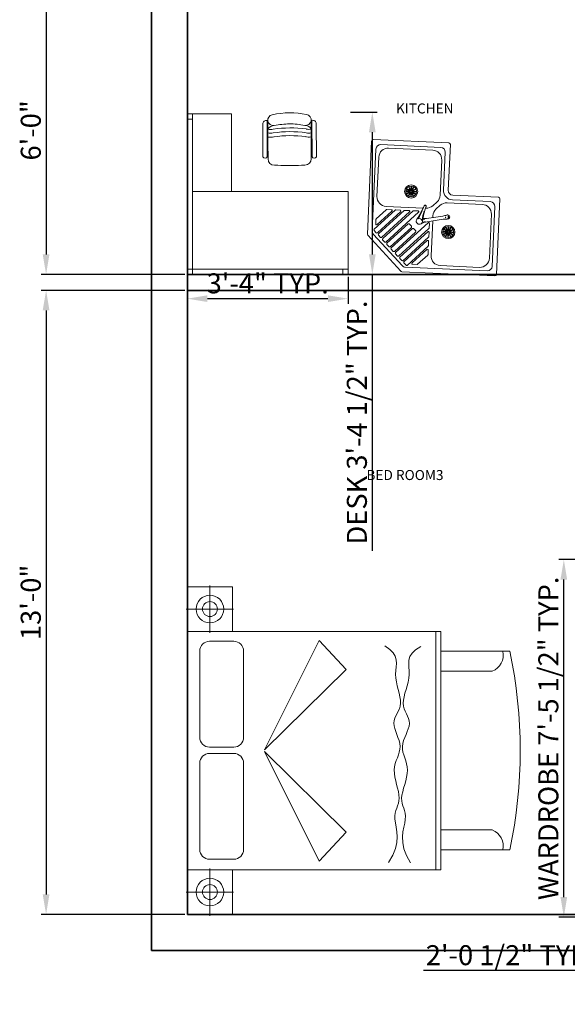
# Model space of a CAD drawing. Units: inches. Extents: x -24887 to 3061, y 1794 to 4919553.
# Tile 8 of 14: x 2721 to 2858, y 1943 to 2190. Entities that reach past the tile are written whole.
import ezdxf

# ---------------------------------------------------------------- set-up
doc = ezdxf.new("R2010")
doc.units = ezdxf.units.IN
for name, color, linetype, lineweight in [('A-ANNO-DIMS', 2, 'Continuous', 18), ('A-AREA-IDEN', 7, 'Continuous', 18), ('A-FLOR-FIXT', 9, 'Continuous', 18), ('A-FURN', 8, 'Continuous', 18), ('wall', 7, 'Continuous', 35)]:
    doc.layers.add(name, color=color, linetype=linetype, lineweight=lineweight)
doc.styles.get("Standard").update_dxf_attribs({"font": 'arial.ttf'})
doc.dimstyles.new('ISO-25', dxfattribs={"dimtxt": 5, "dimasz": 5, "dimexe": 1.25, "dimexo": 0.625, "dimtad": 1, "dimdec": 1, "dimlunit": 3, "dimtxsty": 'Standard', "dimcen": 2.5, "dimadec": 0, "dimazin": 0, "dimtfac": 1, "dimtdec": 1, "dimtmove": 0, "dimatfit": 3, "dimfxl": 1, "dimarcsym": 0})

# ---------------------------------------------------------------- blocks, each defined once
blk = doc.blocks.new('A$C4F543DC7')
for p, q in [((0.0134, 3.35, -0.1688), (3.3134, 3.35, -0.1688)), ((0.4634, 3.35, -0.1688), (0.0134, 3.35, -0.1688)), ((0.0134, 2.896, -0.1688), (0.0134, 3.35, -0.1688)), ((0.0134, 3.35, -0.1688), (0.0134, 2.896, -0.1688)), ((0.2381, 3.1233, -0.4388), (0.2381, 3.3614, -0.4388)), ((0.4634, 3.35, -0.1688), (0.4634, 0.8, -0.1688)), ((2.8634, 3.35, -0.1688), (0.4634, 3.35, -0.1688)), ((0.4634, 2.896, -0.1688), (0.4634, 3.35, -0.1688)), ((2.8634, 0.8, -0.1688), (2.8634, 3.35, -0.1688)), ((2.8634, 3.35, -0.1688), (3.3134, 3.35, -0.1688)), ((2.8634, 2.896, -0.1688), (2.8634, 3.35, -0.1688)), ((3.0888, 3.1233, -0.4388), (3.0888, 3.3614, -0.4388)), ((3.3134, 3.35, -0.1688), (3.3134, 2.896, -0.1688)), ((3.3134, 3.35, -0.1688), (3.3134, 2.896, -0.1688)), ((1.5354, 3.226, -0.1688), (0.6684, 3.226, -0.1688)), ((2.6644, 3.226, -0.1688), (1.7974, 3.226, -0.1688)), ((0.2381, 3.1233, -0.4388), (0, 3.1233, -0.4388)), ((0.2381, 3.1233, -0.4388), (0.4762, 3.1233, -0.4388)), ((0.2381, 3.1233, -0.4388), (0.2381, 2.8852, -0.4388)), ((0.5684, 3.126, -0.1688), (0.5684, 2.884, -0.1688)), ((1.6354, 2.884, -0.1688), (1.6354, 3.126, -0.1688)), ((1.6974, 3.126, -0.1688), (1.6974, 2.884, -0.1688)), ((2.7644, 2.884, -0.1688), (2.7644, 3.126, -0.1688)), ((3.0888, 3.1233, -0.4388), (2.8507, 3.1233, -0.4388)), ((3.0888, 3.1233, -0.4388), (3.0888, 2.8852, -0.4388)), ((3.0888, 3.1233, -0.4388), (3.3269, 3.1233, -0.4388)), ((0.4634, 2.896, -0.1688), (0.0134, 2.896, -0.1688)), ((0.0134, 2.896, -0.1688), (0.4634, 2.896, -0.1688)), ((0.4634, 0.8, -0.1688), (0.4634, 2.896, -0.1688)), ((2.8634, 2.896, -0.1688), (2.8634, 0.8, -0.1688)), ((3.3134, 2.896, -0.1688), (2.8634, 2.896, -0.1688)), ((3.3134, 2.896, -0.1688), (2.8634, 2.896, -0.1688)), ((0.6684, 2.784, -0.1688), (1.5354, 2.784, -0.1688)), ((1.7974, 2.784, -0.1688), (2.6644, 2.784, -0.1688)), ((1.6534, 2.573, -0.1688), (0.5504, 2.025, -0.1688)), ((0.8414, 1.752, -0.1688), (1.6534, 2.573, -0.1688)), ((2.4814, 1.752, -0.1688), (1.6694, 2.573, -0.1688)), ((1.6694, 2.573, -0.1688), (2.7724, 2.025, -0.1688)), ((0.5504, 2.025, -0.1688), (0.8414, 1.752, -0.1688)), ((2.7724, 2.025, -0.1688), (2.4814, 1.752, -0.1688)), ((0.5369, 1.3267, -0.1688), (0.6088, 1.2835, -0.1688)), ((2.6479, 1.2774, -0.1688), (2.683, 1.312, -0.1688)), ((2.683, 1.312, -0.1688), (2.7182, 1.3641, -0.1688)), ((0.6088, 1.2835, -0.1688), (0.6756, 1.2566, -0.1688)), ((0.6756, 1.2566, -0.1688), (0.7373, 1.2428, -0.1688)), ((0.7373, 1.2428, -0.1688), (0.794, 1.239, -0.1688)), ((0.794, 1.239, -0.1688), (0.8457, 1.242, -0.1688)), ((0.8457, 1.242, -0.1688), (0.8925, 1.2489, -0.1688)), ((0.8925, 1.2489, -0.1688), (0.9345, 1.2564, -0.1688)), ((0.9345, 1.2564, -0.1688), (0.9718, 1.2615, -0.1688)), ((0.9718, 1.2615, -0.1688), (1.0044, 1.2617, -0.1688)), ((1.0044, 1.2617, -0.1688), (1.0334, 1.2578, -0.1688)), ((1.0334, 1.2578, -0.1688), (1.0597, 1.2509, -0.1688)), ((1.0597, 1.2509, -0.1688), (1.0842, 1.2424, -0.1688)), ((1.0842, 1.2424, -0.1688), (1.1081, 1.2336, -0.1688)), ((1.1081, 1.2336, -0.1688), (1.1322, 1.2257, -0.1688)), ((1.1316, 1.1872, -0.1688), (1.1573, 1.192, -0.1688)), ((1.1322, 1.2257, -0.1688), (1.1577, 1.2201, -0.1688)), ((1.1573, 1.192, -0.1688), (1.1851, 1.1932, -0.1688)), ((1.1577, 1.2201, -0.1688), (1.1855, 1.218, -0.1688)), ((1.1851, 1.1932, -0.1688), (1.2158, 1.1898, -0.1688)), ((1.1855, 1.218, -0.1688), (1.2163, 1.2204, -0.1688)), ((1.2163, 1.2204, -0.1688), (1.2498, 1.2264, -0.1688)), ((1.2498, 1.2264, -0.1688), (1.2852, 1.2347, -0.1688)), ((1.2852, 1.2347, -0.1688), (1.3218, 1.2441, -0.1688)), ((1.3218, 1.2441, -0.1688), (1.3591, 1.2533, -0.1688)), ((1.3591, 1.2533, -0.1688), (1.3963, 1.2612, -0.1688)), ((1.3963, 1.2612, -0.1688), (1.4328, 1.2664, -0.1688)), ((1.4328, 1.2664, -0.1688), (1.4679, 1.2677, -0.1688)), ((1.4679, 1.2677, -0.1688), (1.501, 1.2643, -0.1688)), ((1.501, 1.2643, -0.1688), (1.5324, 1.257, -0.1688)), ((1.5324, 1.257, -0.1688), (1.5624, 1.2473, -0.1688)), ((1.5624, 1.2473, -0.1688), (1.5915, 1.2365, -0.1688)), ((1.5915, 1.2365, -0.1688), (1.6199, 1.2259, -0.1688)), ((1.6199, 1.2259, -0.1688), (1.6481, 1.2169, -0.1688)), ((1.6481, 1.2169, -0.1688), (1.6765, 1.2108, -0.1688)), ((1.6765, 1.2108, -0.1688), (1.7053, 1.209, -0.1688)), ((1.7053, 1.209, -0.1688), (1.7349, 1.2124, -0.1688)), ((1.7349, 1.2124, -0.1688), (1.7651, 1.2199, -0.1688)), ((1.7651, 1.2199, -0.1688), (1.7955, 1.2301, -0.1688)), ((1.7955, 1.2301, -0.1688), (1.8258, 1.2417, -0.1688)), ((1.8258, 1.2417, -0.1688), (1.8557, 1.2531, -0.1688)), ((1.8557, 1.2531, -0.1688), (1.8849, 1.263, -0.1688)), ((1.8849, 1.263, -0.1688), (1.913, 1.2698, -0.1688)), ((1.913, 1.2698, -0.1688), (1.9397, 1.2722, -0.1688)), ((1.9397, 1.2722, -0.1688), (1.9649, 1.2692, -0.1688)), ((1.9649, 1.2692, -0.1688), (1.989, 1.2617, -0.1688)), ((1.989, 1.2617, -0.1688), (2.0124, 1.2512, -0.1688)), ((2.0124, 1.2512, -0.1688), (2.0359, 1.2391, -0.1688)), ((2.0359, 1.2391, -0.1688), (2.0599, 1.2269, -0.1688)), ((2.0599, 1.2269, -0.1688), (2.0849, 1.216, -0.1688)), ((2.0849, 1.216, -0.1688), (2.1117, 1.2077, -0.1688)), ((2.1117, 1.2077, -0.1688), (2.1407, 1.2037, -0.1688)), ((2.1407, 1.2037, -0.1688), (2.1723, 1.2047, -0.1688)), ((2.1723, 1.2047, -0.1688), (2.2062, 1.21, -0.1688)), ((2.2062, 1.21, -0.1688), (2.242, 1.2182, -0.1688)), ((2.242, 1.2182, -0.1688), (2.2791, 1.2279, -0.1688)), ((2.2791, 1.2279, -0.1688), (2.3173, 1.2378, -0.1688)), ((2.3173, 1.2378, -0.1688), (2.3558, 1.2465, -0.1688)), ((2.3558, 1.2465, -0.1688), (2.3944, 1.2527, -0.1688)), ((2.3944, 1.2527, -0.1688), (2.4325, 1.255, -0.1688)), ((2.4325, 1.255, -0.1688), (2.4698, 1.2529, -0.1688)), ((2.4698, 1.2529, -0.1688), (2.5064, 1.2488, -0.1688)), ((2.5064, 1.2488, -0.1688), (2.5423, 1.2459, -0.1688)), ((2.5423, 1.2459, -0.1688), (2.5777, 1.2476, -0.1688)), ((2.5777, 1.2476, -0.1688), (2.6129, 1.257, -0.1688)), ((2.6129, 1.257, -0.1688), (2.6479, 1.2774, -0.1688)), ((0.5334, 1.105, -0.1688), (0.6067, 1.1458, -0.1688)), ((0.6067, 1.1458, -0.1688), (0.6743, 1.1706, -0.1688)), ((0.6743, 1.1706, -0.1688), (0.7364, 1.1825, -0.1688)), ((0.7364, 1.1825, -0.1688), (0.7931, 1.1846, -0.1688)), ((0.7931, 1.1846, -0.1688), (0.8447, 1.1799, -0.1688)), ((0.8447, 1.1799, -0.1688), (0.8913, 1.1716, -0.1688)), ((0.8913, 1.1716, -0.1688), (0.9331, 1.1628, -0.1688)), ((0.9331, 1.1628, -0.1688), (0.9701, 1.1565, -0.1688)), ((0.9701, 1.1565, -0.1688), (1.0027, 1.1552, -0.1688)), ((1.0027, 1.1552, -0.1688), (1.0318, 1.1582, -0.1688)), ((1.0318, 1.1582, -0.1688), (1.0583, 1.1642, -0.1688)), ((1.0583, 1.1642, -0.1688), (1.0831, 1.172, -0.1688)), ((1.0831, 1.172, -0.1688), (1.1072, 1.18, -0.1688)), ((1.1072, 1.18, -0.1688), (1.1316, 1.1872, -0.1688)), ((1.2158, 1.1898, -0.1688), (1.2491, 1.1828, -0.1688)), ((1.2491, 1.1828, -0.1688), (1.2842, 1.1734, -0.1688)), ((1.2842, 1.1734, -0.1688), (1.3206, 1.1629, -0.1688)), ((1.3206, 1.1629, -0.1688), (1.3575, 1.1524, -0.1688)), ((1.3575, 1.1524, -0.1688), (1.3945, 1.1434, -0.1688)), ((1.3945, 1.1434, -0.1688), (1.4308, 1.1371, -0.1688)), ((1.4308, 1.1371, -0.1688), (1.4658, 1.1347, -0.1688)), ((1.4658, 1.1347, -0.1688), (1.499, 1.137, -0.1688)), ((1.499, 1.137, -0.1688), (1.5306, 1.1433, -0.1688)), ((1.5306, 1.1433, -0.1688), (1.5609, 1.152, -0.1688)), ((1.5609, 1.152, -0.1688), (1.5903, 1.1619, -0.1688)), ((1.5903, 1.1619, -0.1688), (1.6191, 1.1716, -0.1688)), ((1.6191, 1.1716, -0.1688), (1.6475, 1.1797, -0.1688)), ((1.6475, 1.1797, -0.1688), (1.676, 1.1849, -0.1688)), ((1.676, 1.1849, -0.1688), (1.7049, 1.1858, -0.1688)), ((1.7049, 1.1858, -0.1688), (1.7344, 1.1816, -0.1688)), ((1.7344, 1.1816, -0.1688), (1.7643, 1.1731, -0.1688)), ((1.7643, 1.1731, -0.1688), (1.7944, 1.1619, -0.1688)), ((1.7944, 1.1619, -0.1688), (1.8244, 1.1494, -0.1688)), ((1.8244, 1.1494, -0.1688), (1.8539, 1.137, -0.1688)), ((1.8539, 1.137, -0.1688), (1.8827, 1.1263, -0.1688)), ((1.8827, 1.1263, -0.1688), (1.9106, 1.1186, -0.1688)), ((1.9106, 1.1186, -0.1688), (1.9373, 1.1153, -0.1688)), ((1.9373, 1.1153, -0.1688), (1.9625, 1.1176, -0.1688)), ((1.9625, 1.1176, -0.1688), (1.9868, 1.1243, -0.1688)), ((1.9868, 1.1243, -0.1688), (2.0106, 1.134, -0.1688)), ((2.0106, 1.134, -0.1688), (2.0344, 1.1454, -0.1688)), ((2.0344, 1.1454, -0.1688), (2.0588, 1.1568, -0.1688)), ((2.0588, 1.1568, -0.1688), (2.0842, 1.167, -0.1688)), ((2.0842, 1.167, -0.1688), (2.1112, 1.1743, -0.1688)), ((2.1112, 1.1743, -0.1688), (2.1403, 1.1775, -0.1688)), ((2.1403, 1.1775, -0.1688), (2.1718, 1.1755, -0.1688)), ((2.1718, 1.1755, -0.1688), (2.2056, 1.1691, -0.1688)), ((2.2056, 1.1691, -0.1688), (2.2411, 1.1598, -0.1688)), ((2.2411, 1.1598, -0.1688), (2.2779, 1.1489, -0.1688)), ((2.2779, 1.1489, -0.1688), (2.3157, 1.1379, -0.1688)), ((2.3157, 1.1379, -0.1688), (2.354, 1.1279, -0.1688)), ((2.354, 1.1279, -0.1688), (2.3923, 1.1205, -0.1688)), ((2.3923, 1.1205, -0.1688), (2.4304, 1.117, -0.1688)), ((2.4304, 1.117, -0.1688), (2.4677, 1.118, -0.1688)), ((2.4677, 1.118, -0.1688), (2.5043, 1.1209, -0.1688)), ((2.5043, 1.1209, -0.1688), (2.5403, 1.1226, -0.1688)), ((2.5403, 1.1226, -0.1688), (2.5757, 1.1199, -0.1688)), ((2.5757, 1.1199, -0.1688), (2.6106, 1.1094, -0.1688)), ((2.6106, 1.1094, -0.1688), (2.645, 1.0879, -0.1688)), ((2.645, 1.0879, -0.1688), (2.6789, 1.0522, -0.1688)), ((2.6789, 1.0522, -0.1688), (2.7124, 0.999, -0.1688)), ((0.4634, 0.85, -0.1688), (2.8634, 0.85, -0.1688)), ((0.4634, 0.8, -0.1688), (2.8634, 0.8, -0.1688)), ((0.6634, 0.8, -0.1688), (0.4634, 0.8, -0.1688)), ((0.6634, 0.8, -0.1688), (2.6634, 0.8, -0.1688)), ((0.6634, 0.104, -0.1688), (0.6634, 0.8, -0.1688)), ((0.6634, 0.104, -0.1688), (0.6634, 0.8, -0.1688)), ((0.8634, 0.281, -0.1688), (0.8634, 0.8, -0.1688)), ((2.4634, 0.8, -0.1688), (2.4634, 0.281, -0.1688)), ((2.8634, 0.8, -0.1688), (2.6634, 0.8, -0.1688)), ((2.6634, 0.8, -0.1688), (2.6634, 0.104, -0.1688)), ((2.6634, 0.8, -0.1688), (2.6634, 0.104, -0.1688))]:
    blk.add_line(p, q)
for centre, radius in [((0.2381, 3.1233, -0.4388), 0.139), ((0.2381, 3.1233, -0.4388), 0.075), ((3.0888, 3.1233, -0.4388), 0.139), ((3.0888, 3.1233, -0.4388), 0.075)]:
    blk.add_circle(centre, radius)
for centre, radius, start, end in [((0.6684, 3.126, -0.1688), 0.1, 90, 180), ((1.5354, 3.126, -0.1688), 0.1, 0, 90), ((1.7974, 3.126, -0.1688), 0.1, 90, 180), ((2.6644, 3.126, -0.1688), 0.1, 0, 90), ((0.6684, 2.884, -0.1688), 0.1, 180, 270), ((1.5354, 2.884, -0.1688), 0.1, 270, 0), ((1.7974, 2.884, -0.1688), 0.1, 180, 270), ((2.6644, 2.884, -0.1688), 0.1, 270, 0), ((0.6994, 0.3472, -0.1688), 0.1769, 258.2616, 338.03196), ((2.6275, 0.3472, -0.1688), 0.1769, 201.96804, 281.7384), ((1.6634, 4.8597, -0.1688), 4.8597, 258.12517, 281.87483), ((1.6634, 4.8597, -0.1688), 4.8597, 258.12517, 281.87483)]:
    blk.add_arc(centre, radius, start, end)
blk = doc.blocks.new('A$C4E531579')
for p, q in [((222.1, 827.1), (2.9, 607.9)), ((229.1, 830), (820, 830)), ((830, 820), (830, 340)), ((228.6, 791.2), (38.8, 601.4)), ((225.6, 759.9), (211.5, 745.8)), ((388.5, 604.1), (232.7, 759.9)), ((253.9, 788.2), (239.8, 774.1)), ((381.5, 625.3), (239.8, 767)), ((249.9, 800), (770, 800)), ((388.5, 660.7), (261, 788.2)), ((381.5, 681.9), (291.9, 771.5)), ((295.4, 780), (323.7, 780)), ((388.5, 717.2), (327.2, 778.5)), ((720, 780), (470, 780)), ((800, 770), (800, 390)), ((169.1, 703.4), (154.9, 689.2)), ((305.1, 574.4), (176.1, 703.4)), ((197.4, 731.6), (183.2, 717.5)), ((381.5, 512.2), (183.2, 710.4)), ((388.5, 547.5), (204.4, 731.6)), ((381.5, 568.7), (211.5, 738.7)), ((390, 713.7), (390, 685.4)), ((410, 720), (410, 483.9)), ((780, 440), (780, 720)), ((98.4, 632.6), (112.5, 646.8)), ((282.5, 441.5), (98.4, 625.6)), ((317.8, 448.5), (119.6, 646.8)), ((126.6, 660.9), (140.8, 675.1)), ((255.6, 524.9), (126.6, 653.9)), ((276.8, 546.1), (147.9, 675.1)), ((283.9, 553.2), (154.9, 682.1)), ((390, 657.1), (390, 628.8)), ((0, 10), (0, 600.9)), ((30, 60), (30, 580.1)), ((41.8, 576.1), (55.9, 590.2)), ((169.3, 441.5), (41.8, 569)), ((204.7, 448.5), (63, 590.2)), ((70.1, 604.4), (84.2, 618.5)), ((225.9, 441.5), (70.1, 597.3)), ((261.3, 448.5), (91.3, 618.5)), ((305.1, 567.3), (291, 553.2)), ((390, 600.6), (390, 572.3)), ((50, 534.6), (50, 506.3)), ((112.8, 441.5), (51.5, 502.8)), ((148.1, 448.5), (58.5, 538.1)), ((262.7, 524.9), (276.8, 539)), ((390, 544), (390, 515.7)), ((116.3, 440), (144.6, 440)), ((172.9, 440), (201.2, 440)), ((229.4, 440), (257.7, 440)), ((286, 440), (314.3, 440)), ((344.7, 353.4), (324.5, 455.5)), ((344.5, 460.1), (364.9, 357.1)), ((410, 468.8), (410, 466.1)), ((110, 420), (331.5, 420)), ((352.4, 420), (363.9, 420)), ((406.4, 402.4), (432.4, 376.4)), ((427.6, 423.6), (453.6, 397.6)), ((496.1, 380), (720, 380)), ((50, 110), (50, 360)), ((450, 333.9), (450, 110)), ((530, 360), (770, 360)), ((530, 330), (820, 330)), ((470, 300), (470, 60)), ((500, 300), (500, 10)), ((440, 30), (60, 30)), ((390, 50), (110, 50)), ((490, 0), (10, 0))]:
    blk.add_line(p, q)
for centre, radius in [((511.9, 565), 41.9), ((511.9, 565), 34.4), ((511.9, 565), 5.37), ((265, 318.1), 41.9), ((265, 318.1), 34.4), ((265, 318.1), 5.37)]:
    blk.add_circle(centre, radius)
for centre, radius, start, end in [((229.1, 820), 10, 90, 135), ((820, 820), 10, 0, 90), ((229.2, 756.4), 5, 45, 135), ((249.9, 770), 30, 90, 135), ((243.3, 770.5), 5, 135, 225), ((257.5, 784.7), 5, 45, 135), ((295.4, 775), 5, 90, 225), ((323.7, 775), 5, 45, 90), ((470, 720), 60, 90, 180), ((720, 720), 60, 0, 90), ((770, 770), 30, 0, 90), ((158.5, 685.7), 5, 135, 225), ((172.6, 699.8), 5, 45, 135), ((186.7, 714), 5, 135, 225), ((200.9, 728.1), 5, 45, 135), ((215, 742.2), 5, 135, 225), ((385, 713.7), 5, 0, 45), ((101.9, 629.1), 5, 135, 225), ((116, 643.3), 5, 45, 135), ((130.2, 657.4), 5, 135, 225), ((144.3, 671.5), 5, 45, 135), ((385, 685.4), 5, 225, 0), ((385, 628.8), 5, 225, 0), ((385, 657.1), 5, 0, 45), ((10, 600.9), 10, 135, 180), ((60, 580.1), 30, 135, 180), ((45.3, 572.5), 5, 135, 225), ((59.5, 586.7), 5, 45, 135), ((73.6, 600.8), 5, 135, 225), ((87.8, 615), 5, 45, 135), ((301.6, 570.8), 5, 315, 45), ((385, 572.3), 5, 225, 0), ((385, 600.6), 5, 0, 45), ((55, 534.6), 5, 45, 180), ((55, 506.3), 5, 180, 225), ((259.2, 528.4), 5, 225, 315), ((273.3, 542.6), 5, 315, 45), ((287.4, 556.7), 5, 225, 315), ((325.6, 504.4), 20, 52.72293, 268.78568), ((326.2, 504.9), 16.2, 278.92915, 32.15573), ((583, 916.9), 466.4, 238.27092, 250.20216), ((479.5, 750.1), 274.6, 239.9645, 252.02573), ((385, 515.7), 5, 225, 0), ((385, 544), 5, 0, 45), ((116.3, 445), 5, 225, 270), ((144.6, 445), 5, 270, 45), ((172.9, 445), 5, 225, 270), ((201.2, 445), 5, 270, 45), ((229.4, 445), 5, 225, 270), ((257.7, 445), 5, 270, 45), ((286, 445), 5, 225, 270), ((226.1, 437.3), 100, 10.4867, 33.97381), ((314.3, 445), 5, 270, 45), ((296.1, 462.7), 29.3, 9.84672, 38.35374), ((282.9, 16.5), 469.7, 72.94476, 84.83287), ((305.7, 211.8), 277.4, 72.23491, 84.23498), ((368.8, 476.8), 29.3, 168.25085, 191.99309), ((442.8, 478.3), 100, 177.65932, 190.48676), ((470, 466.1), 60, 180, 225), ((422.7, 471.9), 6.64, 252.6444, 68.86421), ((420.8, 471.6), 4.91, 314.25167, 37.23492), ((720, 440), 60, 270, 0), ((110, 360), 60, 90, 180), ((363.9, 360), 60, 45, 90), ((390, 333.9), 60, 0, 45), ((496.1, 440), 60, 225, 270), ((770, 390), 30, 270, 0), ((246.4, 335.2), 100, 355.98426, 10.4867), ((360, 327.2), 13.9, 175.98426, 24.98921), ((359.8, 327.5), 8.12, 180.36355, 342.44433), ((359, 332), 7.59, 72.42297, 131.67578), ((463.2, 375.3), 100, 190.48676, 204.98921), ((530, 300), 60, 90, 180), ((530, 300), 30, 90, 180), ((820, 340), 10, 270, 0), ((110, 110), 60, 180, 270), ((390, 110), 60, 270, 0), ((10, 10), 10, 180, 270), ((60, 60), 30, 180, 270), ((440, 60), 30, 270, 0), ((490, 10), 10, 270, 0)]:
    blk.add_arc(centre, radius, start, end)
at = {"extrusion": (0, -1e-16, -1)}
for centre, major_axis in [((492, 565), (14.5, 0)), ((511.9, 545.1), (0, 14.5))]:
    blk.add_ellipse(centre, major_axis=major_axis, ratio=0.137964, dxfattribs=at)
at = {"extrusion": (-1e-16, -2e-16, -1)}
blk.add_ellipse((494.7, 574.9), major_axis=(12.6, -7.2), ratio=0.137964, dxfattribs=at)
at = {"extrusion": (0, -2e-16, -1)}
for centre, major_axis in [((494.7, 555.1), (12.6, 7.2)), ((529.1, 574.9), (-12.6, -7.2))]:
    blk.add_ellipse(centre, major_axis=major_axis, ratio=0.137964, dxfattribs=at)
at = {"extrusion": (0, 0, -1)}
for centre, major_axis in [((501.9, 582.2), (7.2, -12.6)), ((511.9, 584.9), (0, -14.5)), ((521.8, 547.8), (-7.2, 12.6))]:
    blk.add_ellipse(centre, major_axis=major_axis, ratio=0.137964, dxfattribs=at)
at = {"extrusion": (3e-16, -1e-16, -1)}
blk.add_ellipse((521.8, 582.2), major_axis=(-7.2, -12.6), ratio=0.137964, dxfattribs=at)
at = {"extrusion": (-1e-16, -1e-16, -1)}
blk.add_ellipse((529.1, 555.1), major_axis=(-12.6, 7.2), ratio=0.137964, dxfattribs=at)
at = {"extrusion": (1e-16, -1e-16, -1)}
blk.add_ellipse((531.7, 565), major_axis=(-14.5, 0), ratio=0.137964, dxfattribs=at)
at = {"extrusion": (-3e-16, 1e-16, -1)}
blk.add_ellipse((501.9, 547.8), major_axis=(7.2, 12.6), ratio=0.137964, dxfattribs=at)
for centre, major_axis in [((245.1, 318.1), (14.5, 0)), ((247.8, 328.1), (12.6, -7.2)), ((247.8, 308.2), (12.6, 7.2)), ((255.1, 335.3), (7.2, -12.6)), ((255.1, 300.9), (7.2, 12.6)), ((265, 338), (0, -14.5)), ((265, 298.3), (0, 14.5)), ((274.9, 335.3), (-7.2, -12.6)), ((274.9, 300.9), (-7.2, 12.6)), ((282.2, 328.1), (-12.6, -7.2)), ((282.2, 308.2), (-12.6, 7.2)), ((284.9, 318.1), (-14.5, 0))]:
    blk.add_ellipse(centre, major_axis=major_axis, ratio=0.137964)
blk = doc.blocks.new('DESK-CORNER-WITH-CHAIR')
for p, q in [((0, 40.37), (40.11, 40.37)), ((0, 19.67), (0, 40.37)), ((1.29, 39.07), (1.29, 40.37)), ((38.82, 40.37), (38.82, 19.67)), ((40.11, 40.37), (40.11, 0.26)), ((0, 39.07), (40.11, 39.07)), ((38.82, 19.67), (0, 19.67)), ((29.11, 19.67), (38.82, 19.67)), ((29.11, 0.26), (29.11, 19.67)), ((38.82, 19.67), (38.82, 0.26)), ((10.75, 13.07), (10.91, 13.07)), ((11.62, 13.07), (10.91, 13.07)), ((17.49, 13.1), (18.37, 13.11)), ((7.89, 10.98), (7.93, 2.72)), ((8.97, 10.98), (9.02, 1.91)), ((9.17, 10.98), (9.17, 11.46)), ((9.17, 10.99), (9.18, 9.53)), ((19.98, 11.02), (19.97, 11.52)), ((19.98, 11.02), (19.98, 9.56)), ((20.18, 11.01), (20.22, 1.94)), ((21.26, 11.02), (21.3, 2.76)), ((9.17, 9.52), (9.22, 2.03)), ((19.99, 9.54), (20.03, 2.06)), ((40.11, 0.26), (29.11, 0.26)), ((40.11, 1.55), (38.82, 1.55))]:
    blk.add_line(p, q)
for centre, radius, start, end in [((10.76, 11.47), 1.6, 90.3083, 180.3083), ((14.78, -28.11), 41.3, 86.2317, 94.3849), ((18.38, 11.51), 1.6, 0.3083, 90.3083), ((8.43, 10.73), 0.593, 24.5958, 155.829), ((20.52, 10.77), 0.593, 204.3355, 206.5711), ((20.72, 10.77), 0.593, 24.7876, 156.0208), ((9.82, 2.64), 3.42, 74.7531, 100.4859), ((9.82, 2.64), 2.42, 74.7531, 104.4332), ((14.4, 34.16), 29.46, 262.2773, 278.3393), ((14.4, 34.16), 28.46, 262.2773, 278.3393), ((19.33, 2.69), 3.42, 78.6001, 104.4332), ((19.33, 2.69), 2.42, 73.6429, 104.4332), ((8.75, 2.68), 0.821, 177.6524, 288.8331), ((10.57, 1.77), 1.37, 80.5561, 260.4095), ((10.9, 5.33), 2.21, 220.0354, 267.4848), ((9.82, 1.7), 2.42, 74.7531, 104.4332), ((14.4, 33.22), 29.46, 262.2773, 278.3393), ((14.95, 25.37), 22.63, 259.4369, 269.1516), ((14.03, 25.37), 22.63, 271.465, 281.1797), ((18.3, 5.37), 2.21, 273.1318, 320.9947), ((18.66, 1.82), 1.37, 280.2071, 100.0605), ((19.33, 1.75), 2.42, 73.6429, 104.4332), ((20.48, 2.72), 0.821, 251.7835, 2.9643), ((14.52, 20.73), 20.73, 258.3982, 282.2184)]:
    blk.add_arc(centre, radius, start, end)
blk = doc.blocks.new('*D42')
at = {"layer": 'A-ANNO-DIMS', "color": 0, "lineweight": -2, "transparency": 16777216}
for p, q in [((2869.72, 2054.62), (2855.7, 2054.62)), ((2856.95, 1970.28), (2856.95, 2049.62)), ((2869.72, 1965.28), (2855.7, 1965.28))]:
    blk.add_line(p, q, dxfattribs=at)
at = {"layer": 'A-ANNO-DIMS', "color": 0, "transparency": 16777216}
for points in [[(2856.11, 2049.62), (2857.78, 2049.62), (2856.95, 2054.62)], [(2856.11, 1970.28), (2857.78, 1970.28), (2856.95, 1965.28)]]:
    blk.add_solid(points, dxfattribs=at)
at = {"layer": 'Defpoints', "color": 0, "transparency": 16777216}
for p in [(2856.95, 2054.62), (2870.35, 2054.62), (2870.35, 1965.28)]:
    blk.add_point(p, dxfattribs=at)
at = {"layer": 'A-ANNO-DIMS', "color": 0, "transparency": 16777216, "insert": (2853.73, 2009.95), "char_height": 5, "attachment_point": 5, "rotation": 90}
blk.add_mtext('WARDROBE 7\'-5 1/2" TYP.', dxfattribs=at)
blk = doc.blocks.new('*D43')
at = {"layer": 'A-ANNO-DIMS', "color": 0, "lineweight": -2, "transparency": 16777216}
for p, q in [((2870.35, 1964.65), (2870.35, 1950.63)), ((2894.76, 1964.65), (2894.76, 1950.63)), ((2870.35, 1951.88), (2821.88, 1951.88)), ((2889.76, 1951.88), (2875.35, 1951.88))]:
    blk.add_line(p, q, dxfattribs=at)
at = {"layer": 'A-ANNO-DIMS', "color": 0, "transparency": 16777216}
for points in [[(2875.35, 1952.71), (2875.35, 1951.04), (2870.35, 1951.88)], [(2889.76, 1952.71), (2889.76, 1951.04), (2894.76, 1951.88)]]:
    blk.add_solid(points, dxfattribs=at)
at = {"layer": 'Defpoints', "color": 0, "transparency": 16777216}
for p in [(2870.35, 1965.28), (2894.76, 1965.28), (2870.35, 1951.88)]:
    blk.add_point(p, dxfattribs=at)
at = {"layer": 'A-ANNO-DIMS', "color": 0, "transparency": 16777216, "insert": (2843.62, 1955.09), "char_height": 5, "attachment_point": 5}
blk.add_mtext('2\'-0 1/2" TYP.', dxfattribs=at)
blk = doc.blocks.new('*D48')
at = {"layer": 'A-ANNO-DIMS', "color": 0, "lineweight": -2, "transparency": 16777216}
for p, q in [((2803.66, 2166.46), (2810.36, 2166.46)), ((2809.11, 2161.46), (2809.11, 2130.94)), ((2803.66, 2125.94), (2810.36, 2125.94)), ((2809.11, 2125.94), (2809.11, 2056.85))]:
    blk.add_line(p, q, dxfattribs=at)
at = {"layer": 'A-ANNO-DIMS', "color": 0, "transparency": 16777216}
for points in [[(2808.28, 2161.46), (2809.95, 2161.46), (2809.11, 2166.46)], [(2808.28, 2130.94), (2809.95, 2130.94), (2809.11, 2125.94)]]:
    blk.add_solid(points, dxfattribs=at)
at = {"layer": 'Defpoints', "color": 0, "transparency": 16777216}
for p in [(2803.04, 2166.46), (2803.04, 2125.94), (2809.11, 2125.94)]:
    blk.add_point(p, dxfattribs=at)
at = {"layer": 'A-ANNO-DIMS', "color": 0, "transparency": 16777216, "insert": (2805.9, 2088.9), "char_height": 5, "attachment_point": 5, "rotation": 90}
blk.add_mtext('DESK 3\'-4 1/2" TYP.', dxfattribs=at)
blk = doc.blocks.new('*D49')
at = {"layer": 'A-ANNO-DIMS', "color": 0, "lineweight": -2, "transparency": 16777216}
for p, q in [((2762.93, 2125.32), (2762.93, 2118.61)), ((2803.04, 2125.32), (2803.04, 2118.61)), ((2798.04, 2119.86), (2767.93, 2119.86))]:
    blk.add_line(p, q, dxfattribs=at)
at = {"layer": 'A-ANNO-DIMS', "color": 0, "transparency": 16777216}
for points in [[(2767.93, 2120.7), (2767.93, 2119.03), (2762.93, 2119.86)], [(2798.04, 2120.7), (2798.04, 2119.03), (2803.04, 2119.86)]]:
    blk.add_solid(points, dxfattribs=at)
at = {"layer": 'Defpoints', "color": 0, "transparency": 16777216}
for p in [(2762.93, 2125.94), (2803.04, 2125.94), (2762.93, 2119.86)]:
    blk.add_point(p, dxfattribs=at)
at = {"layer": 'A-ANNO-DIMS', "color": 0, "transparency": 16777216, "insert": (2782.98, 2123.04), "char_height": 5, "attachment_point": 5}
blk.add_mtext('3\'-4" TYP.', dxfattribs=at)
blk = doc.blocks.new('*D104')
at = {"layer": 'A-ANNO-DIMS', "color": 0, "lineweight": -2, "transparency": 16777216}
for p, q in [((2762.3, 2197.94), (2726.38, 2197.94)), ((2727.63, 2192.94), (2727.63, 2130.94)), ((2762.3, 2125.94), (2726.38, 2125.94))]:
    blk.add_line(p, q, dxfattribs=at)
at = {"layer": 'A-ANNO-DIMS', "color": 0, "transparency": 16777216}
for points in [[(2726.79, 2192.94), (2728.46, 2192.94), (2727.63, 2197.94)], [(2726.79, 2130.94), (2728.46, 2130.94), (2727.63, 2125.94)]]:
    blk.add_solid(points, dxfattribs=at)
at = {"layer": 'Defpoints', "color": 0, "transparency": 16777216}
for p in [(2762.93, 2197.94), (2727.63, 2125.94), (2762.93, 2125.94)]:
    blk.add_point(p, dxfattribs=at)
at = {"layer": 'A-ANNO-DIMS', "color": 0, "transparency": 16777216, "insert": (2724.45, 2161.94), "char_height": 5, "attachment_point": 5, "rotation": 90}
blk.add_mtext('6\'-0"', dxfattribs=at)
blk = doc.blocks.new('*D105')
at = {"layer": 'A-ANNO-DIMS', "color": 0, "lineweight": -2, "transparency": 16777216}
for p, q in [((2762.3, 2121.94), (2726.38, 2121.94)), ((2727.63, 2116.94), (2727.63, 1970.94)), ((2762.3, 1965.94), (2726.38, 1965.94))]:
    blk.add_line(p, q, dxfattribs=at)
at = {"layer": 'A-ANNO-DIMS', "color": 0, "transparency": 16777216}
for points in [[(2726.79, 2116.94), (2728.46, 2116.94), (2727.63, 2121.94)], [(2726.79, 1970.94), (2728.46, 1970.94), (2727.63, 1965.94)]]:
    blk.add_solid(points, dxfattribs=at)
at = {"layer": 'Defpoints', "color": 0, "transparency": 16777216}
for p in [(2762.93, 2121.94), (2727.63, 1965.94), (2762.93, 1965.94)]:
    blk.add_point(p, dxfattribs=at)
at = {"layer": 'A-ANNO-DIMS', "color": 0, "transparency": 16777216, "insert": (2724.45, 2043.94), "char_height": 5, "attachment_point": 5, "rotation": 90}
blk.add_mtext('13\'-0"', dxfattribs=at)

msp = doc.modelspace()

# ---------------------------------------------------------------- linework, layer by layer
at = {"layer": 'wall'}
for p, q in [((2753.93, 2436.94), (2753.93, 1956.94)), ((2762.93, 2427.94), (2762.93, 1965.94)), ((2894.93, 2125.94), (2762.93, 2125.94)), ((2894.93, 2121.94), (2762.93, 2121.94)), ((2762.93, 1965.94), (2955.93, 1965.94)), ((2753.93, 1956.94), (2954.95, 1956.94))]:
    msp.add_line(p, q, dxfattribs=at)

# ---------------------------------------------------------------- block references
at = {"layer": 'A-FLOR-FIXT', "xscale": 0.0393700787401575, "yscale": 0.0393700787401575, "zscale": 0.0393700787401575, "rotation": 87.40810793426772}
msp.add_blockref('A$C4E531579', (2840.12, 2125.53), dxfattribs=at)
at = {"layer": 'A-FURN', "rotation": 180}
msp.add_blockref('DESK-CORNER-WITH-CHAIR', (2803.04, 2166.31), dxfattribs=at)
at = {"layer": 'A-FURN', "xscale": 24.81469674658305, "yscale": 24.81469674658305, "zscale": 24.81469674658305, "rotation": 90}
msp.add_blockref('A$C4F543DC7', (2846.05, 1965.61, 4.19), dxfattribs=at)

# ---------------------------------------------------------------- texts
at = {"layer": 'A-AREA-IDEN', "char_height": 2.5, "attachment_point": 1}
for s, insert in [('KITCHEN', (2815.01, 2168.66)), ('BED ROOM3', (2807.65, 2077.02))]:
    msp.add_mtext_dynamic_manual_height_columns(s, width=34.2323, gutter_width=12.5, heights=[0], dxfattribs=dict(at, insert=insert))

# ---------------------------------------------------------------- dimensions: what is measured, and where the dimension line sits
at = {"layer": 'A-ANNO-DIMS'}
for base, p1, p2, picture, middle in [((2727.63, 2125.94), (2762.93, 2197.94), (2762.93, 2125.94), '*D104', (2724.45, 2161.94)), ((2727.63, 1965.94), (2762.93, 2121.94), (2762.93, 1965.94), '*D105', (2724.45, 2043.94))]:
    dim = msp.add_linear_dim(base=base, p1=p1, p2=p2, angle=90, dimstyle='ISO-25', override={"dimdec": 1, "dimlfac": 1, "dimrnd": 0, "dimzin": 1, "dimdsep": 46, "dimlunit": 4, "dimfrac": 2}, dxfattribs=at)
    dim.commit()
    dim.dimension.update_dxf_attribs({"geometry": picture, "text_midpoint": middle})
for base, p1, p2, angle, text, picture, middle in [((2809.11, 2125.94), (2803.04, 2166.46), (2803.04, 2125.94), 270, 'DESK <> TYP.', '*D48', (2805.9, 2088.9)), ((2762.93, 2119.86), (2803.04, 2125.94), (2762.93, 2125.94), 180, '<> TYP.', '*D49', (2782.98, 2123.04)), ((2856.95, 2054.62), (2870.35, 1965.28), (2870.35, 2054.62), 90, 'WARDROBE <> TYP.', '*D42', (2853.73, 2009.95)), ((2870.35, 1951.88), (2894.76, 1965.28), (2870.35, 1965.28), 180, '<> TYP.', '*D43', (2843.62, 1955.09))]:
    dim = msp.add_linear_dim(base=base, p1=p1, p2=p2, angle=angle, text=text, dimstyle='ISO-25', override={"dimdec": 1, "dimlfac": 1, "dimrnd": 0, "dimzin": 1, "dimdsep": 46, "dimlunit": 4, "dimfrac": 2}, dxfattribs=at)
    dim.commit()
    dim.dimension.update_dxf_attribs({"geometry": picture, "text_midpoint": middle})

doc.saveas('drawing.dxf')
